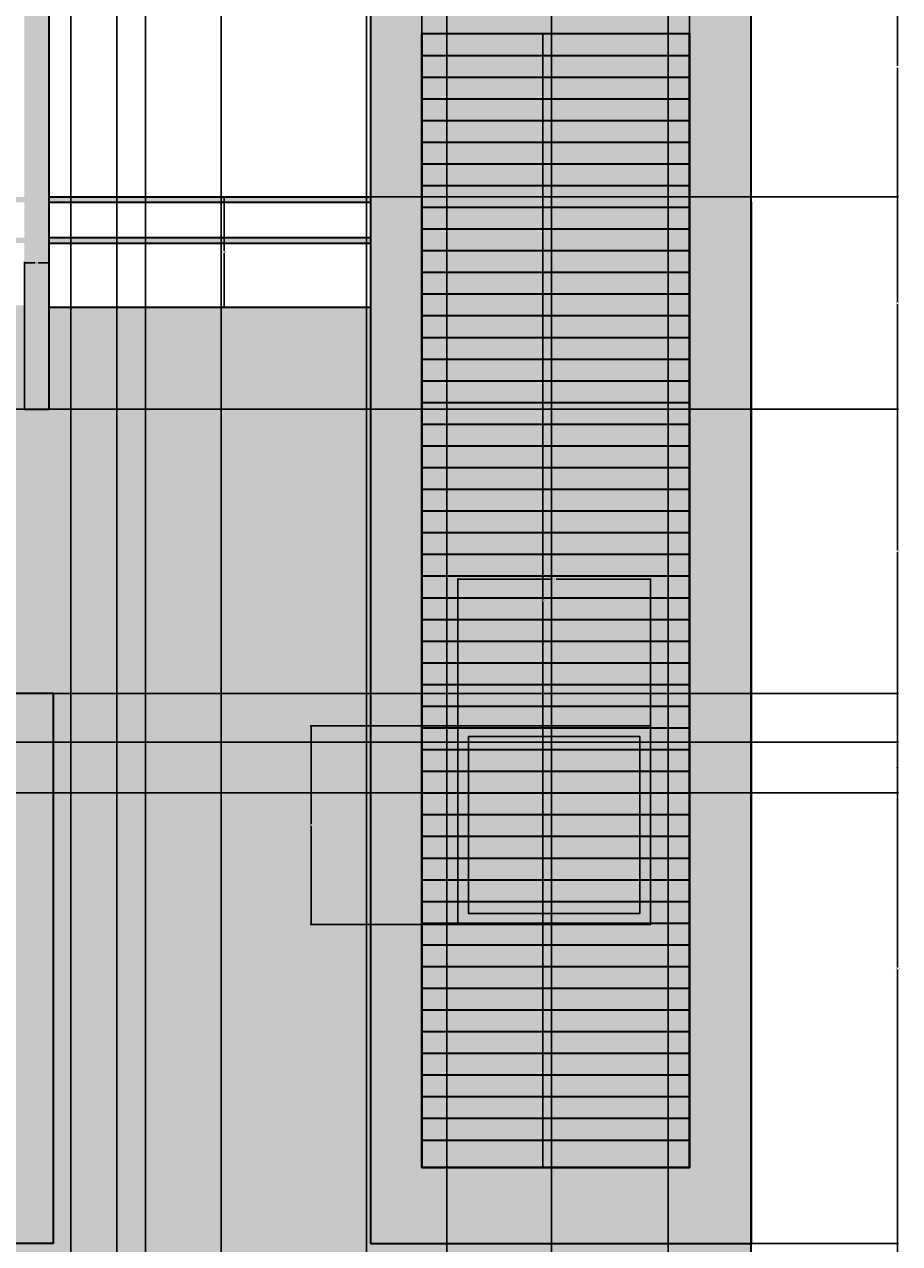
# Model space of a CAD drawing. Units: inches. Extents: x 73 to 607, y 92 to 651.
# Tile 17 of 18: x 446 to 607, y 311 to 536. Entities that reach past the tile are written whole.
import ezdxf

# ---------------------------------------------------------------- set-up
doc = ezdxf.new("R2010")
doc.units = ezdxf.units.IN
doc.header["$MEASUREMENT"] = 0
for name, color, linetype, lineweight in [('A-ANNO-DIMS', 2, 'Continuous', 18), ('A-ELEV', 7, 'Continuous', 35), ('A-ELEV-PATT-BKGD', 252, 'Continuous', 13), ('A-ELEV-PATT-FRAM', 38, 'Continuous', 13), ('A-ELEV-PATT-SHAD', 8, 'Continuous', 13), ('A-ELEV-PATT-WALL', 254, 'Continuous', 13), ('A-ELEV-PATT-WOOD', 32, 'Continuous', 13), ('A-GLAZ', 4, 'Continuous', 25), ('A-GLAZ-PATT', 7, 'Continuous', 13)]:
    doc.layers.add(name, color=color, linetype=linetype, lineweight=lineweight)
doc.styles.get("Standard").update_dxf_attribs({"font": 'arial.ttf'})
doc.dimstyles.get("Standard").update_dxf_attribs({"dimtxt": 0.18, "dimasz": 0.18, "dimexe": 0.18, "dimexo": 0.0625, "dimgap": 0.09, "dimtad": 0, "dimtih": 1, "dimtoh": 1, "dimdec": 4, "dimzin": 0, "dimdsep": 46, "dimtxsty": 'Standard', "dimcen": 0.09, "dimadec": 0, "dimazin": 0, "dimtfac": 1, "dimtdec": 4, "dimtofl": 0, "dimtmove": 0, "dimatfit": 3, "dimfxl": 1, "dimtolj": 1, "dimtzin": 0, "dimarcsym": 0})

# ---------------------------------------------------------------- blocks, each defined once
blk = doc.blocks.new('*D18')
at = {"layer": 'A-ANNO-DIMS', "color": 0, "lineweight": -2, "transparency": 16777216}
for p, q in [((580.16, 311.2), (607.28, 311.2)), ((607.1, 311.02), (607.1, 286.94)), ((607.1, 262.48), (607.1, 286.57)), ((580.16, 262.3), (607.28, 262.3))]:
    blk.add_line(p, q, dxfattribs=at)
at = {"layer": 'A-ANNO-DIMS', "color": 0, "transparency": 16777216}
for points in [[(607.07, 311.02), (607.13, 311.02), (607.1, 311.2)], [(607.07, 262.48), (607.13, 262.48), (607.1, 262.3)]]:
    blk.add_solid(points, dxfattribs=at)
at = {"layer": 'Defpoints', "color": 0, "transparency": 16777216}
for p in [(580.1, 311.2), (607.1, 311.2), (580.1, 262.3)]:
    blk.add_point(p, dxfattribs=at)
at = {"layer": 'A-ANNO-DIMS', "color": 0, "transparency": 16777216, "insert": (607.1, 286.75), "char_height": 0.18, "attachment_point": 5}
blk.add_mtext('\\A1;48.9', dxfattribs=at)
blk = doc.blocks.new('*D19')
at = {"layer": 'A-ANNO-DIMS', "color": 0, "lineweight": -2, "transparency": 16777216}
for p, q in [((451.58, 412.64), (607.28, 412.64)), ((607.1, 412.46), (607.1, 362.1)), ((607.1, 311.38), (607.1, 361.74)), ((580.16, 311.2), (607.28, 311.2))]:
    blk.add_line(p, q, dxfattribs=at)
at = {"layer": 'A-ANNO-DIMS', "color": 0, "transparency": 16777216}
for points in [[(607.07, 412.46), (607.13, 412.46), (607.1, 412.64)], [(607.07, 311.38), (607.13, 311.38), (607.1, 311.2)]]:
    blk.add_solid(points, dxfattribs=at)
at = {"layer": 'Defpoints', "color": 0, "transparency": 16777216}
for p in [(451.52, 412.64), (607.1, 412.64), (580.1, 311.2)]:
    blk.add_point(p, dxfattribs=at)
at = {"layer": 'A-ANNO-DIMS', "color": 0, "transparency": 16777216, "insert": (607.1, 361.92), "char_height": 0.18, "attachment_point": 5}
blk.add_mtext('\\A1;101.43', dxfattribs=at)
blk = doc.blocks.new('*D20')
at = {"layer": 'A-ANNO-DIMS', "color": 0, "lineweight": -2, "transparency": 16777216}
for p, q in [((450.72, 465.06), (607.28, 465.06)), ((607.1, 464.88), (607.1, 439.03)), ((607.1, 412.82), (607.1, 438.67)), ((451.58, 412.64), (607.28, 412.64))]:
    blk.add_line(p, q, dxfattribs=at)
at = {"layer": 'A-ANNO-DIMS', "color": 0, "transparency": 16777216}
for points in [[(607.07, 464.88), (607.13, 464.88), (607.1, 465.06)], [(607.07, 412.82), (607.13, 412.82), (607.1, 412.64)]]:
    blk.add_solid(points, dxfattribs=at)
at = {"layer": 'Defpoints', "color": 0, "transparency": 16777216}
for p in [(450.66, 465.06), (607.1, 465.06), (451.52, 412.64)]:
    blk.add_point(p, dxfattribs=at)
at = {"layer": 'A-ANNO-DIMS', "color": 0, "transparency": 16777216, "insert": (607.1, 438.85), "char_height": 0.18, "attachment_point": 5}
blk.add_mtext('\\A1;52.43', dxfattribs=at)
blk = doc.blocks.new('*D21')
at = {"layer": 'A-ANNO-DIMS', "color": 0, "lineweight": -2, "transparency": 16777216}
for p, q in [((510.03, 504.2), (607.28, 504.2)), ((607.1, 504.02), (607.1, 484.82)), ((607.1, 465.24), (607.1, 484.45)), ((450.72, 465.06), (607.28, 465.06))]:
    blk.add_line(p, q, dxfattribs=at)
at = {"layer": 'A-ANNO-DIMS', "color": 0, "transparency": 16777216}
for points in [[(607.07, 504.02), (607.13, 504.02), (607.1, 504.2)], [(607.07, 465.24), (607.13, 465.24), (607.1, 465.06)]]:
    blk.add_solid(points, dxfattribs=at)
at = {"layer": 'Defpoints', "color": 0, "transparency": 16777216}
for p in [(509.97, 504.2), (607.1, 504.2), (450.66, 465.06)]:
    blk.add_point(p, dxfattribs=at)
at = {"layer": 'A-ANNO-DIMS', "color": 0, "transparency": 16777216, "insert": (607.1, 484.63), "char_height": 0.18, "attachment_point": 5}
blk.add_mtext('\\A1;39.14', dxfattribs=at)
blk = doc.blocks.new('*D22')
at = {"layer": 'A-ANNO-DIMS', "color": 0, "lineweight": -2, "transparency": 16777216}
for p, q in [((580.16, 552.16), (607.28, 552.16)), ((607.1, 551.98), (607.1, 528.36)), ((607.1, 504.38), (607.1, 528)), ((510.03, 504.2), (607.28, 504.2))]:
    blk.add_line(p, q, dxfattribs=at)
at = {"layer": 'A-ANNO-DIMS', "color": 0, "transparency": 16777216}
for points in [[(607.07, 551.98), (607.13, 551.98), (607.1, 552.16)], [(607.07, 504.38), (607.13, 504.38), (607.1, 504.2)]]:
    blk.add_solid(points, dxfattribs=at)
at = {"layer": 'Defpoints', "color": 0, "transparency": 16777216}
for p in [(580.1, 552.16), (607.1, 552.16), (509.97, 504.2)]:
    blk.add_point(p, dxfattribs=at)
at = {"layer": 'A-ANNO-DIMS', "color": 0, "transparency": 16777216, "insert": (607.1, 528.18), "char_height": 0.18, "attachment_point": 5}
blk.add_mtext('\\A1;47.95', dxfattribs=at)
blk = doc.blocks.new('*D25')
at = {"layer": 'A-ANNO-DIMS', "color": 0, "lineweight": -2, "transparency": 16777216}
for p, q in [((509.91, 504.2), (482.79, 504.2)), ((482.97, 504.02), (482.97, 494.21)), ((482.97, 484.04), (482.97, 493.85)), ((509.91, 483.86), (482.79, 483.86))]:
    blk.add_line(p, q, dxfattribs=at)
at = {"layer": 'A-ANNO-DIMS', "color": 0, "transparency": 16777216}
for points in [[(482.94, 504.02), (483, 504.02), (482.97, 504.2)], [(482.94, 484.04), (483, 484.04), (482.97, 483.86)]]:
    blk.add_solid(points, dxfattribs=at)
at = {"layer": 'Defpoints', "color": 0, "transparency": 16777216}
for p in [(482.97, 504.2), (509.97, 504.2), (509.97, 483.86)]:
    blk.add_point(p, dxfattribs=at)
at = {"layer": 'A-ANNO-DIMS', "color": 0, "transparency": 16777216, "insert": (482.97, 494.03), "char_height": 0.18, "attachment_point": 5}
blk.add_mtext('\\A1;20.347', dxfattribs=at)
blk = doc.blocks.new('*D46')
at = {"layer": 'A-ANNO-DIMS', "color": 0, "lineweight": -2, "transparency": 16777216}
for p, q in [((450.6, 552.16), (423.48, 552.16)), ((423.66, 551.98), (423.66, 508.79)), ((423.66, 465.24), (423.66, 508.43)), ((450.6, 465.06), (423.48, 465.06))]:
    blk.add_line(p, q, dxfattribs=at)
at = {"layer": 'A-ANNO-DIMS', "color": 0, "transparency": 16777216}
for points in [[(423.63, 551.98), (423.69, 551.98), (423.66, 552.16)], [(423.63, 465.24), (423.69, 465.24), (423.66, 465.06)]]:
    blk.add_solid(points, dxfattribs=at)
at = {"layer": 'Defpoints', "color": 0, "transparency": 16777216}
for p in [(423.66, 552.16), (450.66, 552.16), (450.66, 465.06)]:
    blk.add_point(p, dxfattribs=at)
at = {"layer": 'A-ANNO-DIMS', "color": 0, "transparency": 16777216, "insert": (423.66, 508.61), "char_height": 0.18, "attachment_point": 5}
blk.add_mtext('\\A1;87.1', dxfattribs=at)
blk = doc.blocks.new('*D47')
at = {"layer": 'A-ANNO-DIMS', "color": 0, "lineweight": -2, "transparency": 16777216}
for p, q in [((446.16, 465.13), (446.16, 492.24)), ((446.34, 492.06), (448.15, 492.06)), ((450.48, 492.06), (448.67, 492.06)), ((450.66, 465.13), (450.66, 492.24))]:
    blk.add_line(p, q, dxfattribs=at)
at = {"layer": 'A-ANNO-DIMS', "color": 0, "transparency": 16777216}
for points in [[(446.34, 492.09), (446.34, 492.03), (446.16, 492.06)], [(450.48, 492.09), (450.48, 492.03), (450.66, 492.06)]]:
    blk.add_solid(points, dxfattribs=at)
at = {"layer": 'Defpoints', "color": 0, "transparency": 16777216}
for p in [(450.66, 492.06), (446.16, 465.06), (450.66, 465.06)]:
    blk.add_point(p, dxfattribs=at)
at = {"layer": 'A-ANNO-DIMS', "color": 0, "transparency": 16777216, "insert": (448.41, 492.06), "char_height": 0.18, "attachment_point": 5}
blk.add_mtext('\\A1;4.5', dxfattribs=at)
blk = doc.blocks.new('*D48')
at = {"layer": 'A-ANNO-DIMS', "color": 0, "lineweight": -2, "transparency": 16777216}
for p, q in [((519.42, 534.37), (519.42, 561.49)), ((519.6, 561.31), (543.75, 561.31)), ((568.54, 561.31), (544.4, 561.31)), ((568.72, 534.37), (568.72, 561.49))]:
    blk.add_line(p, q, dxfattribs=at)
at = {"layer": 'A-ANNO-DIMS', "color": 0, "transparency": 16777216}
for points in [[(519.6, 561.34), (519.6, 561.28), (519.42, 561.31)], [(568.54, 561.34), (568.54, 561.28), (568.72, 561.31)]]:
    blk.add_solid(points, dxfattribs=at)
at = {"layer": 'Defpoints', "color": 0, "transparency": 16777216}
for p in [(568.72, 561.31), (519.42, 534.31), (568.72, 534.31)]:
    blk.add_point(p, dxfattribs=at)
at = {"layer": 'A-ANNO-DIMS', "color": 0, "transparency": 16777216, "insert": (544.07, 561.31), "char_height": 0.18, "attachment_point": 5}
blk.add_mtext('\\A1;49.3', dxfattribs=at)
blk = doc.blocks.new('*D49')
at = {"layer": 'A-ANNO-DIMS', "color": 0, "lineweight": -2, "transparency": 16777216}
for p, q in [((568.66, 534.31), (541.54, 534.31)), ((541.72, 534.13), (541.72, 429.95)), ((541.72, 325.41), (541.72, 429.59)), ((568.66, 325.23), (541.54, 325.23))]:
    blk.add_line(p, q, dxfattribs=at)
at = {"layer": 'A-ANNO-DIMS', "color": 0, "transparency": 16777216}
for points in [[(541.69, 534.13), (541.75, 534.13), (541.72, 534.31)], [(541.69, 325.41), (541.75, 325.41), (541.72, 325.23)]]:
    blk.add_solid(points, dxfattribs=at)
at = {"layer": 'Defpoints', "color": 0, "transparency": 16777216}
for p in [(541.72, 534.31), (568.72, 534.31), (568.72, 325.23)]:
    blk.add_point(p, dxfattribs=at)
at = {"layer": 'A-ANNO-DIMS', "color": 0, "transparency": 16777216, "insert": (541.72, 429.77), "char_height": 0.18, "attachment_point": 5}
blk.add_mtext('\\A1;209.07', dxfattribs=at)
blk = doc.blocks.new('*D50')
at = {"layer": 'A-ANNO-DIMS', "color": 0, "lineweight": -2, "transparency": 16777216}
for p, q in [((526.04, 406.76), (526.04, 433.87)), ((526.22, 433.69), (543.41, 433.69)), ((561.39, 433.69), (544.2, 433.69)), ((561.57, 406.76), (561.57, 433.87))]:
    blk.add_line(p, q, dxfattribs=at)
at = {"layer": 'A-ANNO-DIMS', "color": 0, "transparency": 16777216}
for points in [[(526.22, 433.72), (526.22, 433.66), (526.04, 433.69)], [(561.39, 433.72), (561.39, 433.66), (561.57, 433.69)]]:
    blk.add_solid(points, dxfattribs=at)
at = {"layer": 'Defpoints', "color": 0, "transparency": 16777216}
for p in [(561.57, 433.69), (526.04, 406.69), (561.57, 406.69)]:
    blk.add_point(p, dxfattribs=at)
at = {"layer": 'A-ANNO-DIMS', "color": 0, "transparency": 16777216, "insert": (543.8, 433.69), "char_height": 0.18, "attachment_point": 5}
blk.add_mtext('\\A1;35.53', dxfattribs=at)
blk = doc.blocks.new('*D51')
at = {"layer": 'A-ANNO-DIMS', "color": 0, "lineweight": -2, "transparency": 16777216}
for p, q in [((525.98, 406.69), (498.86, 406.69)), ((499.04, 406.51), (499.04, 388.55)), ((499.04, 370.22), (499.04, 388.19)), ((525.98, 370.04), (498.86, 370.04))]:
    blk.add_line(p, q, dxfattribs=at)
at = {"layer": 'A-ANNO-DIMS', "color": 0, "transparency": 16777216}
for points in [[(499.01, 406.51), (499.07, 406.51), (499.04, 406.69)], [(499.01, 370.22), (499.07, 370.22), (499.04, 370.04)]]:
    blk.add_solid(points, dxfattribs=at)
at = {"layer": 'Defpoints', "color": 0, "transparency": 16777216}
for p in [(499.04, 406.69), (526.04, 406.69), (526.04, 370.04)]:
    blk.add_point(p, dxfattribs=at)
at = {"layer": 'A-ANNO-DIMS', "color": 0, "transparency": 16777216, "insert": (499.04, 388.37), "char_height": 0.18, "attachment_point": 5}
blk.add_mtext('\\A1;36.65', dxfattribs=at)
blk = doc.blocks.new('*D79')
at = {"layer": 'A-ANNO-DIMS', "color": 0, "lineweight": -2, "transparency": 16777216}
for p, q in [((334.73, 403.64), (607.28, 403.64)), ((607.1, 403.46), (607.1, 399.16)), ((607.1, 394.49), (607.1, 398.79)), ((316.35, 394.31), (607.28, 394.31))]:
    blk.add_line(p, q, dxfattribs=at)
at = {"layer": 'A-ANNO-DIMS', "color": 0, "transparency": 16777216}
for points in [[(607.07, 403.46), (607.13, 403.46), (607.1, 403.64)], [(607.07, 394.49), (607.13, 394.49), (607.1, 394.31)]]:
    blk.add_solid(points, dxfattribs=at)
at = {"layer": 'Defpoints', "color": 0, "transparency": 16777216}
for p in [(334.67, 403.64), (316.28, 394.31), (607.1, 394.31)]:
    blk.add_point(p, dxfattribs=at)
at = {"layer": 'A-ANNO-DIMS', "color": 0, "transparency": 16777216, "insert": (607.1, 398.98), "char_height": 0.18, "attachment_point": 5}
blk.add_mtext('\\A1;9.322', dxfattribs=at)
blk = doc.blocks.new('*D103')
at = {"layer": 'A-ANNO-DIMS', "color": 0, "lineweight": -2, "transparency": 16777216}
for p, q in [((454.7, 256.69), (454.7, 650.98)), ((454.88, 650.8), (458.55, 650.8)), ((463, 650.8), (459.34, 650.8)), ((463.18, 243.92), (463.18, 650.98))]:
    blk.add_line(p, q, dxfattribs=at)
at = {"layer": 'A-ANNO-DIMS', "color": 0, "transparency": 16777216}
for points in [[(454.88, 650.83), (454.88, 650.77), (454.7, 650.8)], [(463, 650.83), (463, 650.77), (463.18, 650.8)]]:
    blk.add_solid(points, dxfattribs=at)
at = {"layer": 'Defpoints', "color": 0, "transparency": 16777216}
for p in [(463.18, 650.8), (454.7, 256.63), (463.18, 243.86)]:
    blk.add_point(p, dxfattribs=at)
at = {"layer": 'A-ANNO-DIMS', "color": 0, "transparency": 16777216, "insert": (458.94, 650.8), "char_height": 0.18, "attachment_point": 5}
blk.add_mtext('\\A1;8.475', dxfattribs=at)
blk = doc.blocks.new('*D104')
at = {"layer": 'A-ANNO-DIMS', "color": 0, "lineweight": -2, "transparency": 16777216}
for p, q in [((463.18, 243.92), (463.18, 650.98)), ((463.36, 650.8), (465.44, 650.8)), ((468.3, 650.8), (466.23, 650.8)), ((468.48, 225.79), (468.48, 650.98))]:
    blk.add_line(p, q, dxfattribs=at)
at = {"layer": 'A-ANNO-DIMS', "color": 0, "transparency": 16777216}
for points in [[(463.36, 650.83), (463.36, 650.77), (463.18, 650.8)], [(468.3, 650.83), (468.3, 650.77), (468.48, 650.8)]]:
    blk.add_solid(points, dxfattribs=at)
at = {"layer": 'Defpoints', "color": 0, "transparency": 16777216}
for p in [(468.48, 650.8), (463.18, 243.86), (468.48, 225.73)]:
    blk.add_point(p, dxfattribs=at)
at = {"layer": 'A-ANNO-DIMS', "color": 0, "transparency": 16777216, "insert": (465.83, 650.8), "char_height": 0.18, "attachment_point": 5}
blk.add_mtext('\\A1;5.304', dxfattribs=at)
blk = doc.blocks.new('*D105')
at = {"layer": 'A-ANNO-DIMS', "color": 0, "lineweight": -2, "transparency": 16777216}
for p, q in [((468.48, 225.79), (468.48, 650.98)), ((468.66, 650.8), (475.01, 650.8)), ((482.26, 650.8), (475.92, 650.8)), ((482.44, 246.99), (482.44, 650.98))]:
    blk.add_line(p, q, dxfattribs=at)
at = {"layer": 'A-ANNO-DIMS', "color": 0, "transparency": 16777216}
for points in [[(468.66, 650.83), (468.66, 650.77), (468.48, 650.8)], [(482.26, 650.83), (482.26, 650.77), (482.44, 650.8)]]:
    blk.add_solid(points, dxfattribs=at)
at = {"layer": 'Defpoints', "color": 0, "transparency": 16777216}
for p in [(482.44, 650.8), (482.44, 246.92), (468.48, 225.73)]:
    blk.add_point(p, dxfattribs=at)
at = {"layer": 'A-ANNO-DIMS', "color": 0, "transparency": 16777216, "insert": (475.46, 650.8), "char_height": 0.18, "attachment_point": 5}
blk.add_mtext('\\A1;13.957', dxfattribs=at)
blk = doc.blocks.new('*D106')
at = {"layer": 'A-ANNO-DIMS', "color": 0, "lineweight": -2, "transparency": 16777216}
for p, q in [((482.44, 246.99), (482.44, 650.98)), ((482.62, 650.8), (495.37, 650.8)), ((509.06, 650.8), (496.3, 650.8)), ((509.24, 232.76), (509.24, 650.98))]:
    blk.add_line(p, q, dxfattribs=at)
at = {"layer": 'A-ANNO-DIMS', "color": 0, "transparency": 16777216}
for points in [[(482.62, 650.83), (482.62, 650.77), (482.44, 650.8)], [(509.06, 650.83), (509.06, 650.77), (509.24, 650.8)]]:
    blk.add_solid(points, dxfattribs=at)
at = {"layer": 'Defpoints', "color": 0, "transparency": 16777216}
for p in [(509.24, 650.8), (482.44, 246.92), (509.24, 232.7)]:
    blk.add_point(p, dxfattribs=at)
at = {"layer": 'A-ANNO-DIMS', "color": 0, "transparency": 16777216, "insert": (495.84, 650.8), "char_height": 0.18, "attachment_point": 5}
blk.add_mtext('\\A1;26.797', dxfattribs=at)
blk = doc.blocks.new('*D107')
at = {"layer": 'A-ANNO-DIMS', "color": 0, "lineweight": -2, "transparency": 16777216}
for p, q in [((509.24, 232.76), (509.24, 650.98)), ((509.42, 650.8), (516.18, 650.8)), ((523.85, 650.8), (517.09, 650.8)), ((524.03, 250.33), (524.03, 650.98))]:
    blk.add_line(p, q, dxfattribs=at)
at = {"layer": 'A-ANNO-DIMS', "color": 0, "transparency": 16777216}
for points in [[(509.42, 650.83), (509.42, 650.77), (509.24, 650.8)], [(523.85, 650.83), (523.85, 650.77), (524.03, 650.8)]]:
    blk.add_solid(points, dxfattribs=at)
at = {"layer": 'Defpoints', "color": 0, "transparency": 16777216}
for p in [(524.03, 650.8), (524.03, 250.27), (509.24, 232.7)]:
    blk.add_point(p, dxfattribs=at)
at = {"layer": 'A-ANNO-DIMS', "color": 0, "transparency": 16777216, "insert": (516.63, 650.8), "char_height": 0.18, "attachment_point": 5}
blk.add_mtext('\\A1;14.794', dxfattribs=at)
blk = doc.blocks.new('*D108')
at = {"layer": 'A-ANNO-DIMS', "color": 0, "lineweight": -2, "transparency": 16777216}
for p, q in [((524.03, 250.33), (524.03, 650.98)), ((524.21, 650.8), (533.28, 650.8)), ((543.11, 650.8), (534.05, 650.8)), ((543.29, 226.9), (543.29, 650.98))]:
    blk.add_line(p, q, dxfattribs=at)
at = {"layer": 'A-ANNO-DIMS', "color": 0, "transparency": 16777216}
for points in [[(524.21, 650.83), (524.21, 650.77), (524.03, 650.8)], [(543.11, 650.83), (543.11, 650.77), (543.29, 650.8)]]:
    blk.add_solid(points, dxfattribs=at)
at = {"layer": 'Defpoints', "color": 0, "transparency": 16777216}
for p in [(543.29, 650.8), (524.03, 250.27), (543.29, 226.84)]:
    blk.add_point(p, dxfattribs=at)
at = {"layer": 'A-ANNO-DIMS', "color": 0, "transparency": 16777216, "insert": (533.66, 650.8), "char_height": 0.18, "attachment_point": 5}
blk.add_mtext('\\A1;19.26', dxfattribs=at)
blk = doc.blocks.new('*D109')
at = {"layer": 'A-ANNO-DIMS', "color": 0, "lineweight": -2, "transparency": 16777216}
for p, q in [((543.29, 226.9), (543.29, 650.98)), ((543.47, 650.8), (553.57, 650.8)), ((564.61, 650.8), (554.5, 650.8)), ((564.79, 245.31), (564.79, 650.98))]:
    blk.add_line(p, q, dxfattribs=at)
at = {"layer": 'A-ANNO-DIMS', "color": 0, "transparency": 16777216}
for points in [[(543.47, 650.83), (543.47, 650.77), (543.29, 650.8)], [(564.61, 650.83), (564.61, 650.77), (564.79, 650.8)]]:
    blk.add_solid(points, dxfattribs=at)
at = {"layer": 'Defpoints', "color": 0, "transparency": 16777216}
for p in [(564.79, 650.8), (564.79, 245.25), (543.29, 226.84)]:
    blk.add_point(p, dxfattribs=at)
at = {"layer": 'A-ANNO-DIMS', "color": 0, "transparency": 16777216, "insert": (554.04, 650.8), "char_height": 0.18, "attachment_point": 5}
blk.add_mtext('\\A1;21.493', dxfattribs=at)

msp = doc.modelspace()

# ---------------------------------------------------------------- hatches: boundary and pattern name
at = {"layer": 'A-ELEV-PATT-BKGD'}
h = msp.add_hatch(color=256, dxfattribs=at)
h.dxf.hatch_style = 1
h.paths.add_polyline_path([(321.3008, 479.2042), (312.3008, 479.2042), (312.3008, 478.7576), (312.3008, 412.636), (321.3008, 412.636)])
h.paths.add_polyline_path([(312.3008, 504.7576), (256.4726, 504.7576), (256.4726, 503.4576), (312.3008, 503.4576)], flags=17)
h.paths.add_polyline_path([(321.3008, 543.1576), (321.3008, 552.1576), (320.3257, 552.1576), (312.3008, 552.1576), (256.4726, 552.1576), (256.4726, 543.1576), (312.3008, 543.1576), (312.3008, 479.2042), (321.3008, 479.2042)])
h.paths.add_polyline_path([(451.5214, 412.636), (256.4726, 412.636), (256.4726, 403.636), (442.5214, 403.636), (442.5214, 320.2042), (206.1343, 320.2042), (206.1343, 320.9135), (206.1343, 403.636), (256.4726, 403.636), (256.4726, 412.636), (201.6343, 412.636), (201.6343, 320.9135), (201.6343, 320.2042), (201.6343, 311.2042), (256.4726, 311.2042), (451.5214, 311.2042)])
h.paths.add_polyline_path([(431.07, 258.6914), (369.5339, 258.6914), (369.5339, 247.4054), (396.692, 247.4054), (425.07, 247.4054), (425.07, 194.7312), (396.692, 194.6197), (396.692, 194.5366), (369.5339, 194.5366), (369.5339, 185.6619), (431.07, 185.6619)])
h.paths.add_polyline_path([(580.0983, 262.3024), (451.5214, 262.3024), (451.5214, 143.2042), (580.0983, 143.2042)])
h.paths.add_polyline_path([(454.7049, 174.802), (454.7049, 256.6321), (577.9249, 256.6321), (577.9249, 174.802)], flags=16)
h.paths.add_polyline_path([(465.9716, 191.1416, -1), (473.7874, 191.1416, -1)], flags=0)
h.paths.add_polyline_path([(490.5373, 181.6586, -1), (494.9999, 181.6586, -1)], flags=0)
h.paths.add_polyline_path([(476.2996, 209.8287, -1), (500.5844, 209.8287, -1)], flags=0)
h.paths.add_polyline_path([(505.3326, 194.7675, -1), (512.5843, 194.7675, -1)], flags=0)
h.paths.add_polyline_path([(520.9613, 186.679, -1), (526.544, 186.679, -1)], flags=0)
h.paths.add_polyline_path([(466.8103, 225.7267, -1), (470.1573, 225.7267, -1)], flags=0)
h.paths.add_polyline_path([(527.1059, 203.6926, -1), (536.0311, 203.6926, -1)], flags=0)
h.paths.add_polyline_path([(504.775, 232.6995, -1), (513.7002, 232.6995, -1)], flags=0)
h.paths.add_polyline_path([(546.9241, 183.611, -1), (554.7336, 183.611, -1)], flags=0)
h.paths.add_polyline_path([(459.5544, 243.856, -1), (466.8061, 243.856, -1)], flags=0)
h.paths.add_polyline_path([(476.3045, 246.924, -1), (488.5767, 246.924, -1)], flags=0)
h.paths.add_polyline_path([(529.9044, 226.8424, -1), (556.68, 226.8424, -1)], flags=0)
h.paths.add_polyline_path([(554.1814, 203.9716, -1), (561.4331, 203.9716, -1)], flags=0)
h.paths.add_polyline_path([(567.8561, 193.3729, -1), (570.6475, 193.3729, -1)], flags=0)
h.paths.add_polyline_path([(522.3584, 250.271, -1), (525.7053, 250.271, -1)], flags=0)
h.paths.add_polyline_path([(561.9965, 245.2506, -1), (567.5748, 245.2506, -1)], flags=0)
h.paths.add_polyline_path([(347.8686, 194.5366), (341.8686, 194.5366), (341.8686, 194.5452), (314.0144, 194.5452), (314.0144, 188.5452), (347.8686, 188.5452)])
h.paths.add_polyline_path([(347.8686, 253.4054), (314.0144, 253.4054), (314.0144, 247.4054), (341.8686, 247.4054), (347.8686, 247.4054)])
h.paths.add_polyline_path([(304.3559, 253.4054), (298.3559, 253.4054), (298.3559, 188.5452), (304.3559, 188.5452)])
h.paths.add_polyline_path([(450.6603, 552.1576), (369.9727, 552.1576), (369.9727, 479.2042), (374.4727, 479.2042), (374.4727, 547.6576), (446.1603, 547.6576), (446.1603, 479.2042), (450.6603, 479.2042)])
h.paths.add_polyline_path([(374.4727, 479.2042), (369.9727, 479.2042), (369.9727, 465.0632), (374.4727, 465.0632)])
h.paths.add_polyline_path([(450.6603, 479.2042), (446.1603, 479.2042), (446.1603, 465.0632), (450.6603, 465.0632)])
h.paths.add_polyline_path([(256.4726, 281.6039), (109.0983, 281.6039), (100.0983, 281.6039), (100.0983, 167.2042), (100.0983, 143.2042), (109.0983, 143.2042), (109.0983, 167.2042), (109.0983, 272.6039), (256.4726, 272.6039)])
at = {"layer": 'A-ELEV-PATT-FRAM'}
h = msp.add_hatch(color=256, dxfattribs=at)
h.dxf.hatch_style = 1
h.paths.add_polyline_path([(528.0397, 394.3065), (526.0397, 394.3065), (526.0397, 370.0444), (561.5694, 370.0444), (561.5694, 394.3065), (559.5694, 394.3065), (559.5694, 372.0444), (528.0397, 372.0444)])
h.paths.add_polyline_path([(528.0397, 398.3065), (526.0397, 398.3065), (526.0397, 394.3065), (528.0397, 394.3065)])
h.paths.add_polyline_path([(528.0397, 404.6944), (559.5694, 404.6944), (559.5694, 398.3065), (561.5694, 398.3065), (561.5694, 406.6944), (526.0397, 406.6944), (526.0397, 398.3065), (528.0397, 398.3065)])
h.paths.add_polyline_path([(561.5694, 398.3065), (559.5694, 398.3065), (559.5694, 394.3065), (561.5694, 394.3065)])
at = {"layer": 'A-ELEV-PATT-SHAD'}
h = msp.add_hatch(color=256, dxfattribs=at)
h.dxf.hatch_style = 1
h.paths.add_polyline_path([(451.5214, 412.636), (256.4726, 412.636), (256.4726, 403.636), (442.5214, 403.636), (442.5214, 320.2042), (206.1343, 320.2042), (206.1343, 320.9135), (206.1343, 403.636), (256.4726, 403.636), (256.4726, 412.636), (201.6343, 412.636), (201.6343, 320.9135), (201.6343, 320.2042), (201.6343, 311.2042), (256.4726, 311.2042), (451.5214, 311.2042)])
h.paths.add_polyline_path([(580.0983, 262.3024), (451.5214, 262.3024), (451.5214, 143.2042), (580.0983, 143.2042)])
h.paths.add_polyline_path([(454.7049, 174.802), (454.7049, 256.6321), (577.9249, 256.6321), (577.9249, 174.802)], flags=16)
h.paths.add_polyline_path([(465.9716, 191.1416, -1), (473.7874, 191.1416, -1)], flags=0)
h.paths.add_polyline_path([(490.5373, 181.6586, -1), (494.9999, 181.6586, -1)], flags=0)
h.paths.add_polyline_path([(476.2996, 209.8287, -1), (500.5844, 209.8287, -1)], flags=0)
h.paths.add_polyline_path([(505.3326, 194.7675, -1), (512.5843, 194.7675, -1)], flags=0)
h.paths.add_polyline_path([(520.9613, 186.679, -1), (526.544, 186.679, -1)], flags=0)
h.paths.add_polyline_path([(466.8103, 225.7267, -1), (470.1573, 225.7267, -1)], flags=0)
h.paths.add_polyline_path([(527.1059, 203.6926, -1), (536.0311, 203.6926, -1)], flags=0)
h.paths.add_polyline_path([(459.5544, 243.856, -1), (466.8061, 243.856, -1)], flags=0)
h.paths.add_polyline_path([(504.775, 232.6995, -1), (513.7002, 232.6995, -1)], flags=0)
h.paths.add_polyline_path([(476.3045, 246.924, -1), (488.5767, 246.924, -1)], flags=0)
h.paths.add_polyline_path([(546.9241, 183.611, -1), (554.7336, 183.611, -1)], flags=0)
h.paths.add_polyline_path([(529.9044, 226.8424, -1), (556.68, 226.8424, -1)], flags=0)
h.paths.add_polyline_path([(554.1814, 203.9716, -1), (561.4331, 203.9716, -1)], flags=0)
h.paths.add_polyline_path([(522.3584, 250.271, -1), (525.7053, 250.271, -1)], flags=0)
h.paths.add_polyline_path([(567.8561, 193.3729, -1), (570.6475, 193.3729, -1)], flags=0)
h.paths.add_polyline_path([(561.9965, 245.2506, -1), (567.5748, 245.2506, -1)], flags=0)
h.paths.add_polyline_path([(431.07, 258.6914), (369.5339, 258.6914), (369.5339, 247.4054), (396.692, 247.4054), (425.07, 247.4054), (425.07, 194.7312), (396.692, 194.6197), (396.692, 194.5366), (369.5339, 194.5366), (369.5339, 185.6619), (431.07, 185.6619)])
h.paths.add_polyline_path([(347.8686, 253.4054), (314.0144, 253.4054), (314.0144, 247.4054), (341.8686, 247.4054), (347.8686, 247.4054)])
h.paths.add_polyline_path([(304.3559, 253.4054), (298.3559, 253.4054), (298.3559, 188.5452), (304.3559, 188.5452)])
h.paths.add_polyline_path([(347.8686, 194.5366), (341.8686, 194.5366), (341.8686, 194.5452), (314.0144, 194.5452), (314.0144, 188.5452), (347.8686, 188.5452)])
at = {"layer": 'A-ELEV-PATT-WALL'}
h = msp.add_hatch(color=256, dxfattribs=at)
h.dxf.hatch_style = 1
h.paths.add_polyline_path([(509.9692, 483.857), (450.6603, 483.857), (450.6603, 465.0632), (446.1603, 465.0632), (446.1603, 484.2142), (374.4727, 484.2142), (374.4727, 465.0632), (369.9727, 465.0632), (369.9727, 484.2142), (321.3008, 484.2142), (321.3008, 412.636), (451.5214, 412.636), (451.5214, 311.2042), (314.0144, 311.2042), (314.0144, 253.4054), (347.8686, 253.4054), (347.8686, 247.4054), (369.5339, 247.4054), (369.5339, 258.6914), (431.07, 258.6914), (431.07, 185.6619), (369.5339, 185.6619), (369.5339, 194.5366), (347.8686, 194.5366), (347.8686, 188.5452), (314.0144, 188.5452), (314.0144, 143.2042), (451.5214, 143.2042), (451.5214, 262.3024), (580.0983, 262.3024), (580.0983, 311.2042), (509.9692, 311.2042)])
h.paths.add_polyline_path([(304.3559, 311.2042), (256.4726, 311.2042), (256.4726, 167.2042), (256.4726, 143.2042), (304.3559, 143.2042), (304.3559, 188.5452), (298.3559, 188.5452), (298.3559, 253.4054), (304.3559, 253.4054)])
at = {"layer": 'A-ELEV-PATT-WOOD'}
h = msp.add_hatch(color=256, dxfattribs=at)
h.dxf.hatch_style = 1
h.paths.add_polyline_path([(580.0983, 552.1576), (509.9692, 552.1576), (509.9692, 311.2042), (580.0983, 311.2042)])
h.paths.add_polyline_path([(568.7235, 534.3065), (568.7235, 325.2318), (519.4225, 325.2318), (519.4225, 534.3065)], flags=16)
h.paths.add_polyline_path([(526.0397, 406.6944), (561.5694, 406.6944), (561.5694, 370.0444), (526.0397, 370.0444)], flags=0)
h.paths.add_polyline_path([(528.0397, 404.6944), (559.5694, 404.6944), (559.5694, 372.0444), (528.0397, 372.0444)], flags=0)
h.paths.add_polyline_path([(568.7235, 534.3065), (519.4225, 534.3065), (519.4225, 530.3065), (568.7235, 530.3065)], flags=0)
h.paths.add_polyline_path([(568.7235, 530.3065), (519.4225, 530.3065), (519.4225, 526.3065), (568.7235, 526.3065)], flags=0)
h = msp.add_hatch(color=256, dxfattribs=at)
h.dxf.hatch_style = 1
h.paths.add_polyline_path([(568.7235, 534.3065), (519.4225, 534.3065), (519.4225, 530.3065), (568.7235, 530.3065)])
h.paths.add_polyline_path([(568.7235, 530.3065), (519.4225, 530.3065), (519.4225, 526.3065), (568.7235, 526.3065)])
h.paths.add_polyline_path([(568.7235, 526.3065), (519.4225, 526.3065), (519.4225, 522.3065), (568.7235, 522.3065)])
h.paths.add_polyline_path([(568.7235, 522.3065), (519.4225, 522.3065), (519.4225, 518.3065), (568.7235, 518.3065)])
h.paths.add_polyline_path([(568.7235, 518.3065), (519.4225, 518.3065), (519.4225, 514.3065), (568.7235, 514.3065)])
h.paths.add_polyline_path([(568.7235, 514.3065), (519.4225, 514.3065), (519.4225, 510.3065), (568.7235, 510.3065)])
h.paths.add_polyline_path([(568.7235, 510.3065), (519.4225, 510.3065), (519.4225, 506.3065), (568.7235, 506.3065)])
h.paths.add_polyline_path([(568.7235, 506.3065), (519.4225, 506.3065), (519.4225, 502.3065), (568.7235, 502.3065)])
h.paths.add_polyline_path([(568.7235, 502.3065), (519.4225, 502.3065), (519.4225, 498.3065), (568.7235, 498.3065)])
h.paths.add_polyline_path([(568.7235, 498.3065), (519.4225, 498.3065), (519.4225, 494.3065), (568.7235, 494.3065)])
h.paths.add_polyline_path([(568.7235, 494.3065), (519.4225, 494.3065), (519.4225, 490.3065), (568.7235, 490.3065)])
h.paths.add_polyline_path([(568.7235, 490.3065), (519.4225, 490.3065), (519.4225, 486.3065), (568.7235, 486.3065)])
h.paths.add_polyline_path([(568.7235, 486.3065), (519.4225, 486.3065), (519.4225, 482.3065), (568.7235, 482.3065)])
h.paths.add_polyline_path([(568.7235, 482.3065), (519.4225, 482.3065), (519.4225, 478.3065), (568.7235, 478.3065)])
h.paths.add_polyline_path([(568.7235, 474.3065), (519.4225, 474.3065), (519.4225, 470.3065), (568.7235, 470.3065)])
h = msp.add_hatch(color=256, dxfattribs=at)
h.dxf.hatch_style = 1
h.paths.add_polyline_path([(568.7235, 478.3065), (519.4225, 478.3065), (519.4225, 474.3065), (568.7235, 474.3065)])
h.paths.add_polyline_path([(568.7235, 470.3065), (519.4225, 470.3065), (519.4225, 466.3065), (568.7235, 466.3065)])
h.paths.add_polyline_path([(568.7235, 466.3065), (519.4225, 466.3065), (519.4225, 462.3065), (568.7235, 462.3065)])
h.paths.add_polyline_path([(568.7235, 462.3065), (519.4225, 462.3065), (519.4225, 458.3065), (568.7235, 458.3065)])
h.paths.add_polyline_path([(568.7235, 458.3065), (519.4225, 458.3065), (519.4225, 454.3065), (568.7235, 454.3065)])
h.paths.add_polyline_path([(568.7235, 454.3065), (519.4225, 454.3065), (519.4225, 450.3065), (568.7235, 450.3065)])
h.paths.add_polyline_path([(568.7235, 450.3065), (519.4225, 450.3065), (519.4225, 446.3065), (568.7235, 446.3065)])
h.paths.add_polyline_path([(568.7235, 446.3065), (519.4225, 446.3065), (519.4225, 442.3065), (568.7235, 442.3065)])
h.paths.add_polyline_path([(568.7235, 442.3065), (519.4225, 442.3065), (519.4225, 438.3065), (568.7235, 438.3065)])
h.paths.add_polyline_path([(568.7235, 438.3065), (519.4225, 438.3065), (519.4225, 434.3065), (568.7235, 434.3065)])
h.paths.add_polyline_path([(568.7235, 434.3065), (519.4225, 434.3065), (519.4225, 430.3065), (568.7235, 430.3065)])
h.paths.add_polyline_path([(568.7235, 430.3065), (519.4225, 430.3065), (519.4225, 426.3065), (568.7235, 426.3065)])
h.paths.add_polyline_path([(568.7235, 426.3065), (519.4225, 426.3065), (519.4225, 422.3065), (568.7235, 422.3065)])
h.paths.add_polyline_path([(568.7235, 422.3065), (519.4225, 422.3065), (519.4225, 418.3065), (568.7235, 418.3065)])
h.paths.add_polyline_path([(568.7235, 418.3065), (519.4225, 418.3065), (519.4225, 414.3065), (568.7235, 414.3065)])
h.paths.add_polyline_path([(568.7235, 414.3065), (519.4225, 414.3065), (519.4225, 410.3065), (568.7235, 410.3065)])
h.paths.add_polyline_path([(526.0397, 398.3065), (519.4225, 398.3065), (519.4225, 394.3065), (526.0397, 394.3065)])
h.paths.add_polyline_path([(526.0397, 402.3065), (519.4225, 402.3065), (519.4225, 398.3065), (526.0397, 398.3065)])
h.paths.add_polyline_path([(526.0397, 406.3065), (519.4225, 406.3065), (519.4225, 402.3065), (526.0397, 402.3065)])
h.paths.add_polyline_path([(568.7235, 406.3065), (561.5694, 406.3065), (561.5694, 402.3065), (568.7235, 402.3065)])
h.paths.add_polyline_path([(568.7235, 410.3065), (519.4225, 410.3065), (519.4225, 406.3065), (526.0397, 406.3065), (526.0397, 406.6944), (561.5694, 406.6944), (561.5694, 406.3065), (568.7235, 406.3065)])
h.paths.add_polyline_path([(568.7235, 402.3065), (561.5694, 402.3065), (561.5694, 398.3065), (568.7235, 398.3065)])
h.paths.add_polyline_path([(568.7235, 398.3065), (561.5694, 398.3065), (561.5694, 394.3065), (568.7235, 394.3065)])
h.paths.add_polyline_path([(568.7235, 394.3065), (561.5694, 394.3065), (561.5694, 390.3065), (568.7235, 390.3065)])
h.paths.add_polyline_path([(568.7235, 390.3065), (561.5694, 390.3065), (561.5694, 386.3065), (568.7235, 386.3065)])
h.paths.add_polyline_path([(568.7235, 386.3065), (561.5694, 386.3065), (561.5694, 382.3065), (568.7235, 382.3065)])
h.paths.add_polyline_path([(568.7235, 382.3065), (561.5694, 382.3065), (561.5694, 378.3065), (568.7235, 378.3065)])
h.paths.add_polyline_path([(568.7235, 378.3065), (561.5694, 378.3065), (561.5694, 374.3065), (568.7235, 374.3065)])
h.paths.add_polyline_path([(568.7235, 374.3065), (561.5694, 374.3065), (561.5694, 370.3065), (568.7235, 370.3065)])
h.paths.add_polyline_path([(526.0397, 378.3065), (519.4225, 378.3065), (519.4225, 374.3065), (526.0397, 374.3065)])
h.paths.add_polyline_path([(526.0397, 374.3065), (519.4225, 374.3065), (519.4225, 370.3065), (526.0397, 370.3065)])
h.paths.add_polyline_path([(526.0397, 382.3065), (519.4225, 382.3065), (519.4225, 378.3065), (526.0397, 378.3065)])
h.paths.add_polyline_path([(526.0397, 386.3065), (519.4225, 386.3065), (519.4225, 382.3065), (526.0397, 382.3065)])
h.paths.add_polyline_path([(526.0397, 394.3065), (519.4225, 394.3065), (519.4225, 390.3065), (526.0397, 390.3065)])
h.paths.add_polyline_path([(526.0397, 390.3065), (519.4225, 390.3065), (519.4225, 386.3065), (526.0397, 386.3065)])
h.paths.add_polyline_path([(568.7235, 370.3065), (561.5694, 370.3065), (561.5694, 370.0444), (526.0397, 370.0444), (526.0397, 370.3065), (519.4225, 370.3065), (519.4225, 366.3065), (568.7235, 366.3065)])
h.paths.add_polyline_path([(568.7235, 366.3065), (519.4225, 366.3065), (519.4225, 362.3065), (568.7235, 362.3065)])
h.paths.add_polyline_path([(568.7235, 362.3065), (519.4225, 362.3065), (519.4225, 358.3065), (568.7235, 358.3065)])
h.paths.add_polyline_path([(568.7235, 358.3065), (519.4225, 358.3065), (519.4225, 354.3065), (568.7235, 354.3065)])
h.paths.add_polyline_path([(568.7235, 354.3065), (519.4225, 354.3065), (519.4225, 350.3065), (568.7235, 350.3065)])
h.paths.add_polyline_path([(568.7235, 350.3065), (519.4225, 350.3065), (519.4225, 346.3065), (568.7235, 346.3065)])
h.paths.add_polyline_path([(568.7235, 346.3065), (519.4225, 346.3065), (519.4225, 342.3065), (568.7235, 342.3065)])
h.paths.add_polyline_path([(568.7235, 342.3065), (519.4225, 342.3065), (519.4225, 338.3065), (568.7235, 338.3065)])
h.paths.add_polyline_path([(568.7235, 338.3065), (519.4225, 338.3065), (519.4225, 334.3065), (568.7235, 334.3065)])
h.paths.add_polyline_path([(568.7235, 334.3065), (519.4225, 334.3065), (519.4225, 330.3065), (568.7235, 330.3065)])
h.paths.add_polyline_path([(568.7235, 330.3065), (519.4225, 330.3065), (519.4225, 325.2318), (568.7235, 325.2318)])
at = {"layer": 'A-GLAZ-PATT'}
h = msp.add_hatch(color=256, dxfattribs=at)
h.dxf.hatch_style = 1
h.paths.add_polyline_path([(369.9727, 496.6899), (321.3008, 496.6899), (321.3008, 495.6899), (369.9727, 495.6899)])
h.paths.add_polyline_path([(394.7799, 496.6899), (374.4727, 496.6899), (374.4727, 495.6899), (394.7799, 495.6899)])
h.paths.add_polyline_path([(446.1603, 496.6899), (394.7799, 496.6899), (394.7799, 495.6899), (446.1603, 495.6899)])
h.paths.add_polyline_path([(446.1603, 504.2042), (394.7799, 504.2042), (394.7799, 503.2042), (446.1603, 503.2042)])
h.paths.add_polyline_path([(369.9727, 504.2042), (321.3008, 504.2042), (321.3008, 503.2042), (369.9727, 503.2042)])
h.paths.add_polyline_path([(394.7799, 504.2042), (374.4727, 504.2042), (374.4727, 503.2042), (394.7799, 503.2042)])
h.paths.add_polyline_path([(509.9692, 504.2042), (450.6603, 504.2042), (450.6603, 503.2042), (509.9692, 503.2042)])
h.paths.add_polyline_path([(509.9692, 496.6899), (450.6603, 496.6899), (450.6603, 495.6899), (509.9692, 495.6899)])
h.paths.add_polyline_path([(409.515, 342.1009), (338.6695, 342.1009), (338.6695, 341.1009), (409.515, 341.1009)])
h.paths.add_polyline_path([(442.5214, 338.0025), (338.6695, 338.0025), (338.6695, 337.0025), (442.5214, 337.0025)])
h.paths.add_polyline_path([(442.5214, 332.9397), (338.6695, 332.9397), (338.6695, 331.9397), (442.5214, 331.9397)])
h = msp.add_hatch(color=256, dxfattribs=at)
h.dxf.hatch_style = 1
h.set_gradient(color1=(0, 0, 255))
h.paths.add_polyline_path([(559.5694, 404.6944), (528.0397, 404.6944), (528.0397, 372.0444), (559.5694, 372.0444)])

# ---------------------------------------------------------------- linework, layer by layer
at = {"layer": 'A-ELEV'}
for p, q in [((450.6603, 552.1576), (450.6603, 465.0632)), ((519.4225, 534.3065), (519.4225, 530.3065)), ((519.4225, 534.3065), (519.4225, 325.2318)), ((568.7235, 325.2318), (568.7235, 534.3065)), ((519.4225, 530.3065), (568.7235, 530.3065)), ((519.4225, 526.3065), (568.7235, 526.3065)), ((519.4225, 522.3065), (568.7235, 522.3065)), ((519.4225, 518.3065), (568.7235, 518.3065)), ((519.4225, 514.3065), (568.7235, 514.3065)), ((519.4225, 510.3065), (568.7235, 510.3065)), ((519.4225, 506.3065), (568.7235, 506.3065)), ((450.6603, 504.2042), (509.9692, 504.2042)), ((450.6603, 503.2042), (509.9692, 503.2042)), ((519.4225, 502.3065), (568.7235, 502.3065)), ((580.0983, 503.2042), (580.0983, 455.2042)), ((519.4225, 498.3065), (568.7235, 498.3065)), ((450.6603, 496.6899), (509.9692, 496.6899)), ((450.6603, 495.6899), (509.9692, 495.6899)), ((519.4225, 494.3065), (568.7235, 494.3065)), ((519.4225, 490.3065), (568.7235, 490.3065)), ((519.4225, 486.3065), (568.7235, 486.3065)), ((450.6603, 483.857), (509.9692, 483.857)), ((519.4225, 482.3065), (568.7235, 482.3065)), ((519.4225, 478.3065), (568.7235, 478.3065)), ((519.4225, 474.3065), (568.7235, 474.3065)), ((519.4225, 470.3065), (568.7235, 470.3065)), ((519.4225, 466.3065), (568.7235, 466.3065)), ((446.1603, 465.0632), (450.6603, 465.0632)), ((519.4225, 462.3065), (568.7235, 462.3065)), ((519.4225, 458.3065), (568.7235, 458.3065)), ((519.4225, 454.3065), (568.7235, 454.3065)), ((580.0983, 455.2042), (580.0983, 311.2042)), ((519.4225, 450.3065), (568.7235, 450.3065)), ((519.4225, 446.3065), (568.7235, 446.3065)), ((519.4225, 442.3065), (568.7235, 442.3065)), ((519.4225, 438.3065), (568.7235, 438.3065)), ((519.4225, 434.3065), (568.7235, 434.3065)), ((519.4225, 430.3065), (568.7235, 430.3065)), ((519.4225, 426.3065), (568.7235, 426.3065)), ((519.4225, 426.3065), (568.7235, 426.3065)), ((519.4225, 422.3065), (568.7235, 422.3065)), ((519.4225, 418.3065), (568.7235, 418.3065)), ((519.4225, 414.3065), (568.7235, 414.3065)), ((451.5214, 412.636), (201.6343, 412.636)), ((451.5214, 311.2042), (451.5214, 412.636)), ((519.4225, 410.3065), (568.7235, 410.3065)), ((519.4225, 406.3065), (568.7235, 406.3065)), ((519.4225, 402.3065), (568.7235, 402.3065)), ((519.4225, 398.3065), (568.7235, 398.3065)), ((519.4225, 394.3065), (568.7235, 394.3065)), ((519.4225, 390.3065), (568.7235, 390.3065)), ((519.4225, 386.3065), (568.7235, 386.3065)), ((519.4225, 382.3065), (568.7235, 382.3065)), ((519.4225, 378.3065), (568.7235, 378.3065)), ((519.4225, 374.3065), (568.7235, 374.3065)), ((519.4225, 370.3065), (568.7235, 370.3065)), ((519.4225, 366.3065), (568.7235, 366.3065)), ((519.4225, 362.3065), (568.7235, 362.3065)), ((519.4225, 358.3065), (568.7235, 358.3065)), ((519.4225, 354.3065), (568.7235, 354.3065)), ((519.4225, 350.3065), (568.7235, 350.3065)), ((519.4225, 346.3065), (568.7235, 346.3065)), ((519.4225, 342.3065), (568.7235, 342.3065)), ((519.4225, 338.3065), (568.7235, 338.3065)), ((519.4225, 334.3065), (568.7235, 334.3065)), ((519.4225, 330.3065), (568.7235, 330.3065)), ((519.4225, 325.2318), (568.7235, 325.2318)), ((451.5214, 311.2042), (256.4726, 311.2042)), ((580.0983, 167.2042), (580.0983, 311.2042))]:
    msp.add_line(p, q, dxfattribs=at)
for points in [[(509.9692, 311.2042), (580.0983, 311.2042), (580.0983, 552.1576), (509.9692, 552.1576)], [(519.4225, 534.3065), (568.7235, 534.3065), (568.7235, 325.2318), (519.4225, 325.2318)]]:
    msp.add_lwpolyline(points, close=True, dxfattribs=at)
at = {"layer": 'A-GLAZ'}
for points in [[(526.0397, 406.6944), (561.5694, 406.6944), (561.5694, 370.0444), (526.0397, 370.0444)], [(528.0397, 404.6944), (559.5694, 404.6944), (559.5694, 372.0444), (528.0397, 372.0444)]]:
    msp.add_lwpolyline(points, close=True, dxfattribs=at)

# ---------------------------------------------------------------- dimensions: what is measured, and where the dimension line sits
at = {"layer": 'A-ANNO-DIMS'}
for base, p1, p2, override, picture, middle in [((463.1802, 650.801), (454.7049, 256.6321), (463.1802, 243.856), {"dimdec": 3, "dimlfac": 1, "dimrnd": 0, "dimzin": 0, "dimdsep": 46, "dimlunit": 2}, '*D103', (458.9425, 650.801)), ((468.4838, 650.801), (463.1802, 243.856), (468.4838, 225.7267), {"dimdec": 3, "dimlfac": 1, "dimrnd": 0, "dimzin": 0, "dimdsep": 46, "dimlunit": 2}, '*D104', (465.832, 650.801)), ((482.4406, 650.801), (468.4838, 225.7267), (482.4406, 246.924), {"dimdec": 3, "dimlfac": 1, "dimrnd": 0, "dimzin": 0, "dimdsep": 46, "dimlunit": 2}, '*D105', (475.4622, 650.801)), ((509.2376, 650.801), (482.4406, 246.924), (509.2376, 232.6995), {"dimdec": 3, "dimlfac": 1, "dimrnd": 0, "dimzin": 0, "dimdsep": 46, "dimlunit": 2}, '*D106', (495.8391, 650.801)), ((524.0318, 650.801), (509.2376, 232.6995), (524.0318, 250.271), {"dimdec": 3, "dimlfac": 1, "dimrnd": 0, "dimzin": 0, "dimdsep": 46, "dimlunit": 2}, '*D107', (516.6347, 650.801)), ((543.2922, 650.801), (524.0318, 250.271), (543.2922, 226.8424), {"dimdec": 2, "dimlfac": 1, "dimrnd": 0, "dimzin": 0, "dimdsep": 46, "dimlunit": 2}, '*D108', (533.662, 650.801)), ((564.7856, 650.801), (543.2922, 226.8424), (564.7856, 245.2506), {"dimdec": 3, "dimlfac": 1, "dimrnd": 0, "dimzin": 0, "dimdsep": 46, "dimlunit": 2}, '*D109', (554.0389, 650.801)), ((568.7235, 561.3065), (519.4225, 534.3065), (568.7235, 534.3065), {"dimdec": 1, "dimlfac": 1, "dimrnd": 0, "dimzin": 0, "dimdsep": 46, "dimlunit": 2}, '*D48', (544.073, 561.3065)), ((450.6603, 492.0632), (446.1603, 465.0632), (450.6603, 465.0632), {"dimdec": 1, "dimlfac": 1, "dimrnd": 0, "dimzin": 0, "dimdsep": 46, "dimlunit": 2}, '*D47', (448.4103, 492.0632)), ((561.5694, 433.6944), (526.0397, 406.6944), (561.5694, 406.6944), {"dimdec": 2, "dimlfac": 1, "dimrnd": 0, "dimzin": 0, "dimdsep": 46, "dimlunit": 2}, '*D50', (543.8046, 433.6944))]:
    dim = msp.add_linear_dim(base=base, p1=p1, p2=p2, dimstyle='Standard', override=override, dxfattribs=at)
    dim.commit()
    dim.dimension.update_dxf_attribs({"geometry": picture, "text_midpoint": middle})
for base, p1, p2, override, picture, middle in [((423.6603, 552.1576), (450.6603, 465.0632), (450.6603, 552.1576), {"dimdec": 1, "dimlfac": 1, "dimrnd": 0, "dimzin": 0, "dimdsep": 46, "dimlunit": 2}, '*D46', (423.6603, 508.6104)), ((607.0983, 552.1576), (509.9692, 504.2042), (580.0983, 552.1576), {"dimdec": 2, "dimlfac": 1, "dimrnd": 0, "dimzin": 0, "dimdsep": 46, "dimlunit": 2}, '*D22', (607.0983, 528.1809)), ((541.7235, 534.3065), (568.7235, 325.2318), (568.7235, 534.3065), {"dimdec": 2, "dimlfac": 1, "dimrnd": 0, "dimzin": 0, "dimdsep": 46, "dimlunit": 2}, '*D49', (541.7235, 429.7692)), ((607.0983, 504.2042), (450.6603, 465.0632), (509.9692, 504.2042), {"dimdec": 2, "dimlfac": 1, "dimrnd": 0, "dimzin": 0, "dimdsep": 46, "dimlunit": 2}, '*D21', (607.0983, 484.6337)), ((482.9692, 504.2042), (509.9692, 483.857), (509.9692, 504.2042), {"dimdec": 3, "dimlfac": 1, "dimrnd": 0, "dimzin": 0, "dimdsep": 46, "dimlunit": 2}, '*D25', (482.9692, 494.0306)), ((607.0983, 465.0632), (451.5214, 412.636), (450.6603, 465.0632), {"dimdec": 2, "dimlfac": 1, "dimrnd": 0, "dimzin": 0, "dimdsep": 46, "dimlunit": 2}, '*D20', (607.0983, 438.8496)), ((607.0983, 412.636), (580.0983, 311.2042), (451.5214, 412.636), {"dimdec": 2, "dimlfac": 1, "dimrnd": 0, "dimzin": 0, "dimdsep": 46, "dimlunit": 2}, '*D19', (607.0983, 361.9201)), ((499.0397, 406.6944), (526.0397, 370.0444), (526.0397, 406.6944), {"dimdec": 2, "dimlfac": 1, "dimrnd": 0, "dimzin": 0, "dimdsep": 46, "dimlunit": 2}, '*D51', (499.0397, 388.3694)), ((607.0983, 394.3141), (334.6695, 403.636), (316.2836, 394.3141), {"dimdec": 3, "dimlfac": 1, "dimrnd": 0, "dimzin": 0, "dimdsep": 46, "dimlunit": 2}, '*D79', (607.0983, 398.9751)), ((607.0983, 311.2042), (580.0983, 262.3024), (580.0983, 311.2042), {"dimdec": 1, "dimlfac": 1, "dimrnd": 0, "dimzin": 0, "dimdsep": 46, "dimlunit": 2}, '*D18', (607.0983, 286.7533))]:
    dim = msp.add_linear_dim(base=base, p1=p1, p2=p2, angle=90, dimstyle='Standard', override=override, dxfattribs=at)
    dim.commit()
    dim.dimension.update_dxf_attribs({"geometry": picture, "text_midpoint": middle})

doc.saveas('drawing.dxf')
